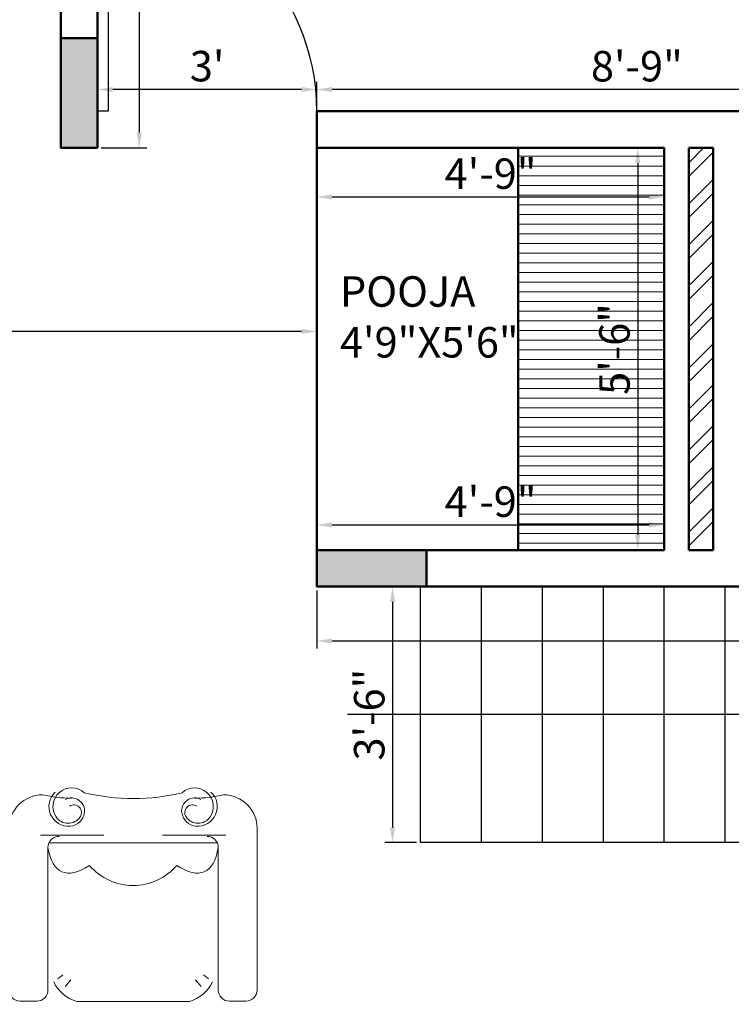
# Model space of a CAD drawing. Units: inches. Extents: x 3064 to 19385, y 846 to 15425.
# Tile 85 of 108: x 7228 to 7345, y 1112 to 1273. Entities that reach past the tile are written whole.
import ezdxf

# ---------------------------------------------------------------- set-up
doc = ezdxf.new("R2010")
doc.units = ezdxf.units.IN
for name, color, linetype, lineweight in [('A-ANNO-DIMS', 2, 'Continuous', 18), ('A-AREA-IDEN', 3, 'Continuous', 18), ('A-COLS', 1, 'Continuous', 35), ('A-DOOR', 3, 'Continuous', 25), ('A-FLOR-STRS', 2, 'Continuous', 25), ('A-FURN', 8, 'Continuous', 18), ('A-FURN-PATT', 252, 'Continuous', 13), ('A-WALL', 7, 'Continuous', 50)]:
    doc.layers.add(name, color=color, linetype=linetype, lineweight=lineweight)
doc.styles.get("Standard").update_dxf_attribs({"font": 'arial.ttf'})
doc.dimstyles.new('ISO-25', dxfattribs={"dimtxt": 9, "dimasz": 2.5, "dimexe": 1.25, "dimexo": 0.625, "dimtad": 1, "dimdec": 1, "dimlunit": 3, "dimtxsty": 'Standard', "dimcen": 2.5, "dimadec": 0, "dimazin": 0, "dimtfac": 1, "dimtdec": 1, "dimtmove": 0, "dimatfit": 3, "dimfxl": 1, "dimarcsym": 0})

# ---------------------------------------------------------------- blocks, each defined once
blk = doc.blocks.new('*U3')
for p, q in [((0, 0), (0, -6)), ((36, 0), (36, -6))]:
    blk.add_line(p, q)
blk.add_lwpolyline([(0, 0), (0, 36), (1.75, 36), (1.75, 0)], close=True)
blk.add_arc((0, 0), 36, 0, 90)
blk = doc.blocks.new('*D281')
at = {"layer": 'A-ANNO-DIMS', "color": 0, "lineweight": -2, "transparency": 16777216}
for p, q in [((7276.71, 1258.96), (7276.71, 1263.17)), ((7379.21, 1261.92), (7279.21, 1261.92)), ((7381.71, 1258.96), (7381.71, 1263.17))]:
    blk.add_line(p, q, dxfattribs=at)
at = {"layer": 'A-ANNO-DIMS', "color": 0, "transparency": 16777216}
for points in [[(7279.21, 1262.33), (7279.21, 1261.5), (7276.71, 1261.92)], [(7379.21, 1262.33), (7379.21, 1261.5), (7381.71, 1261.92)]]:
    blk.add_solid(points, dxfattribs=at)
at = {"layer": 'Defpoints', "color": 0, "transparency": 16777216}
for p in [(7276.71, 1261.92), (7276.71, 1258.34), (7381.71, 1258.34)]:
    blk.add_point(p, dxfattribs=at)
at = {"layer": 'A-ANNO-DIMS', "color": 0, "transparency": 16777216, "insert": (7329.21, 1265.09), "char_height": 5, "attachment_point": 5}
blk.add_mtext('8\'-9"', dxfattribs=at)
blk = doc.blocks.new('*D282')
at = {"layer": 'A-ANNO-DIMS', "color": 0, "lineweight": -2, "transparency": 16777216}
for p, q in [((7240.71, 1258.96), (7240.71, 1263.17)), ((7274.21, 1261.92), (7243.21, 1261.92)), ((7276.71, 1258.96), (7276.71, 1263.17))]:
    blk.add_line(p, q, dxfattribs=at)
at = {"layer": 'A-ANNO-DIMS', "color": 0, "transparency": 16777216}
for points in [[(7243.21, 1262.33), (7243.21, 1261.5), (7240.71, 1261.92)], [(7274.21, 1262.33), (7274.21, 1261.5), (7276.71, 1261.92)]]:
    blk.add_solid(points, dxfattribs=at)
at = {"layer": 'Defpoints', "color": 0, "transparency": 16777216}
for p in [(7240.71, 1261.92), (7240.71, 1258.34), (7276.71, 1258.34)]:
    blk.add_point(p, dxfattribs=at)
at = {"layer": 'A-ANNO-DIMS', "color": 0, "transparency": 16777216, "insert": (7258.71, 1265.1), "char_height": 5, "attachment_point": 5}
blk.add_mtext("3'", dxfattribs=at)
blk = doc.blocks.new('*D275')
at = {"layer": 'A-ANNO-DIMS', "color": 0, "lineweight": -2, "transparency": 16777216}
for p, q in [((7241.33, 1390.34), (7248.82, 1390.34)), ((7247.57, 1387.84), (7247.57, 1254.84)), ((7241.33, 1252.34), (7248.82, 1252.34))]:
    blk.add_line(p, q, dxfattribs=at)
at = {"layer": 'A-ANNO-DIMS', "color": 0, "transparency": 16777216}
for points in [[(7247.15, 1387.84), (7247.99, 1387.84), (7247.57, 1390.34)], [(7247.15, 1254.84), (7247.99, 1254.84), (7247.57, 1252.34)]]:
    blk.add_solid(points, dxfattribs=at)
at = {"layer": 'Defpoints', "color": 0, "transparency": 16777216}
for p in [(7240.71, 1390.34), (7240.71, 1252.34), (7247.57, 1252.34)]:
    blk.add_point(p, dxfattribs=at)
at = {"layer": 'A-ANNO-DIMS', "color": 0, "transparency": 16777216, "insert": (7244.39, 1321.34), "char_height": 5, "attachment_point": 5, "rotation": 90}
blk.add_mtext('11\'-6"', dxfattribs=at)
blk = doc.blocks.new('*D276')
at = {"layer": 'A-ANNO-DIMS', "color": 0, "lineweight": -2, "transparency": 16777216}
for p, q in [((7276.71, 1251.71), (7276.71, 1243.03)), ((7333.71, 1251.71), (7333.71, 1243.03)), ((7279.21, 1244.28), (7331.21, 1244.28))]:
    blk.add_line(p, q, dxfattribs=at)
at = {"layer": 'A-ANNO-DIMS', "color": 0, "transparency": 16777216}
for points in [[(7279.21, 1244.7), (7279.21, 1243.86), (7276.71, 1244.28)], [(7331.21, 1244.7), (7331.21, 1243.86), (7333.71, 1244.28)]]:
    blk.add_solid(points, dxfattribs=at)
at = {"layer": 'Defpoints', "color": 0, "transparency": 16777216}
for p in [(7276.71, 1252.34), (7333.71, 1252.34), (7333.71, 1244.28)]:
    blk.add_point(p, dxfattribs=at)
at = {"layer": 'A-ANNO-DIMS', "color": 0, "transparency": 16777216, "insert": (7305.21, 1247.46), "char_height": 5, "attachment_point": 5}
blk.add_mtext('4\'-9"', dxfattribs=at)
blk = doc.blocks.new('*D277')
at = {"layer": 'A-ANNO-DIMS', "color": 0, "lineweight": -2, "transparency": 16777216}
for p, q in [((7333.08, 1252.34), (7328.11, 1252.34)), ((7329.36, 1249.84), (7329.36, 1188.84)), ((7333.08, 1186.34), (7328.11, 1186.34))]:
    blk.add_line(p, q, dxfattribs=at)
at = {"layer": 'A-ANNO-DIMS', "color": 0, "transparency": 16777216}
for points in [[(7328.94, 1249.84), (7329.77, 1249.84), (7329.36, 1252.34)], [(7328.94, 1188.84), (7329.77, 1188.84), (7329.36, 1186.34)]]:
    blk.add_solid(points, dxfattribs=at)
at = {"layer": 'Defpoints', "color": 0, "transparency": 16777216}
for p in [(7333.71, 1252.34), (7329.36, 1186.34), (7333.71, 1186.34)]:
    blk.add_point(p, dxfattribs=at)
at = {"layer": 'A-ANNO-DIMS', "color": 0, "transparency": 16777216, "insert": (7326.18, 1219.34), "char_height": 5, "attachment_point": 5, "rotation": 90}
blk.add_mtext('5\'-6"', dxfattribs=at)
blk = doc.blocks.new('*D283')
at = {"layer": 'A-ANNO-DIMS', "color": 0, "lineweight": -2, "transparency": 16777216}
for p, q in [((7276.71, 1186.96), (7276.71, 1191.72)), ((7333.71, 1186.96), (7333.71, 1191.72)), ((7279.21, 1190.47), (7331.21, 1190.47))]:
    blk.add_line(p, q, dxfattribs=at)
at = {"layer": 'A-ANNO-DIMS', "color": 0, "transparency": 16777216}
for points in [[(7279.21, 1190.88), (7279.21, 1190.05), (7276.71, 1190.47)], [(7331.21, 1190.88), (7331.21, 1190.05), (7333.71, 1190.47)]]:
    blk.add_solid(points, dxfattribs=at)
at = {"layer": 'Defpoints', "color": 0, "transparency": 16777216}
for p in [(7333.71, 1190.47), (7276.71, 1186.34), (7333.71, 1186.34)]:
    blk.add_point(p, dxfattribs=at)
at = {"layer": 'A-ANNO-DIMS', "color": 0, "transparency": 16777216, "insert": (7305.21, 1193.64), "char_height": 5, "attachment_point": 5}
blk.add_mtext('4\'-9"', dxfattribs=at)
blk = doc.blocks.new('*D238')
at = {"layer": 'A-ANNO-DIMS', "color": 0, "lineweight": -2, "transparency": 16777216}
for p, q in [((7276.71, 1179.71), (7276.71, 1170.17)), ((7435.71, 1179.71), (7435.71, 1170.17)), ((7279.21, 1171.42), (7433.21, 1171.42))]:
    blk.add_line(p, q, dxfattribs=at)
at = {"layer": 'A-ANNO-DIMS', "color": 0, "transparency": 16777216}
for points in [[(7279.21, 1171.84), (7279.21, 1171.01), (7276.71, 1171.42)], [(7433.21, 1171.84), (7433.21, 1171.01), (7435.71, 1171.42)]]:
    blk.add_solid(points, dxfattribs=at)
at = {"layer": 'Defpoints', "color": 0, "transparency": 16777216}
for p in [(7276.71, 1180.34), (7435.71, 1180.34), (7435.71, 1171.42)]:
    blk.add_point(p, dxfattribs=at)
at = {"layer": 'A-ANNO-DIMS', "color": 0, "transparency": 16777216, "insert": (7356.21, 1174.6), "char_height": 5, "attachment_point": 5}
blk.add_mtext('13\'-3"', dxfattribs=at)
blk = doc.blocks.new('*D239')
at = {"layer": 'A-ANNO-DIMS', "color": 0, "lineweight": -2, "transparency": 16777216}
for p, q in [((7105.71, 1222.85), (7105.71, 1223.48)), ((7276.71, 1222.85), (7276.71, 1223.48)), ((7274.21, 1222.23), (7108.21, 1222.23))]:
    blk.add_line(p, q, dxfattribs=at)
at = {"layer": 'A-ANNO-DIMS', "color": 0, "transparency": 16777216}
for points in [[(7108.21, 1222.64), (7108.21, 1221.81), (7105.71, 1222.23)], [(7274.21, 1222.64), (7274.21, 1221.81), (7276.71, 1222.23)]]:
    blk.add_solid(points, dxfattribs=at)
at = {"layer": 'Defpoints', "color": 0, "transparency": 16777216}
for p in [(7105.71, 1222.23), (7105.71, 1222.23), (7276.71, 1222.23)]:
    blk.add_point(p, dxfattribs=at)
at = {"layer": 'A-ANNO-DIMS', "color": 0, "transparency": 16777216, "insert": (7191.21, 1225.4), "char_height": 5, "attachment_point": 5}
blk.add_mtext('14\'-3"', dxfattribs=at)
blk = doc.blocks.new('*D260')
at = {"layer": 'A-ANNO-DIMS', "color": 0, "lineweight": -2, "transparency": 16777216}
for p, q in [((7293.08, 1180.34), (7287.88, 1180.34)), ((7289.13, 1177.84), (7289.13, 1140.84)), ((7293.08, 1138.34), (7287.88, 1138.34))]:
    blk.add_line(p, q, dxfattribs=at)
at = {"layer": 'A-ANNO-DIMS', "color": 0, "transparency": 16777216}
for points in [[(7288.71, 1177.84), (7289.54, 1177.84), (7289.13, 1180.34)], [(7288.71, 1140.84), (7289.54, 1140.84), (7289.13, 1138.34)]]:
    blk.add_solid(points, dxfattribs=at)
at = {"layer": 'Defpoints', "color": 0, "transparency": 16777216}
for p in [(7293.71, 1180.34), (7289.13, 1138.34), (7293.71, 1138.34)]:
    blk.add_point(p, dxfattribs=at)
at = {"layer": 'A-ANNO-DIMS', "color": 0, "transparency": 16777216, "insert": (7285.95, 1159.34), "char_height": 5, "attachment_point": 5, "rotation": 90}
blk.add_mtext('3\'-6"', dxfattribs=at)
blk = doc.blocks.new('sofa-34')
at = {"color": 0, "linetype": 'ByBlock'}
for p, q in [((-0.026, 0.9238), (-0.1, 0.9238)), ((0.657, 0.9252), (0.1531, 0.9252)), ((0.8361, 0.9238), (0.9101, 0.9238)), ((-0.15, 0.15), (-0.15, 0.8738)), ((0.024, 0.2361), (0.024, 0.8738)), ((0.05, 0.8375), (0.05, 0.8379)), ((0.1006, 0.8574), (0.1265, 0.8286)), ((0.7096, 0.8574), (0.6837, 0.8286)), ((0.7601, 0.8375), (0.7601, 0.8379)), ((0.7602, 0.8375), (0.7601, 0.8379)), ((0.7861, 0.2361), (0.7861, 0.8738)), ((0.9601, 0.15), (0.9601, 0.8738)), ((0.0903, 0.8062), (0.0682, 0.8242)), ((0.7199, 0.8062), (0.742, 0.8242)), ((-0.01, 0.1801), (0.2738, 0.1801)), ((0.0289, 0.2145), (0.7812, 0.2145)), ((0.8201, 0.1801), (0.5364, 0.1801))]:
    blk.add_line(p, q, dxfattribs=at)
blk.add_arc((0.4051, 0.1479), 0.2579, 40.7983, 139.2017, dxfattribs=at)
at = {"color": 0, "linetype": 'ByBlock', "extrusion": (0, 0, -1)}
for centre, major_axis, ratio, start_param, end_param in [((-0.1, 0.8738), (0.0354, 0.0354), 1, 3.926992, 5.497787), ((-0.026, 0.8738), (-0.0354, 0.0354), 1, 0.785398, 2.356196), ((0.1997, 0.7661), (0.1173, 0.1173), 1, 4.372209, 5.213218), ((0.6105, 0.7661), (0.1173, 0.1173), 1, -0.500829, 0.34018), ((0.5004, -0.5869), (-0.4145, 0.931), 0.264583, -0.381915, 0.387685), ((0.074, 0.2361), (-0.0354, 0.0354), 1, 3.926991, 5.497788), ((0, 0.15), (0.1061, 0.1061), 1, 2.356194, 3.926992), ((0.1167, 0.0525), (-0.0624, 0.0624), 1, 4.675944, 7.152385), ((0.1183, 0.0712), (0.0491, 0.0491), 1, -0.701597, 0.659711), ((0.1299, 0.0524), (-0.059, 0.059), 1, 3.186406, 6.094039), ((0.1144, 0.0629), (-0.0458, 0.0458), 1, 6.094039, 8.043134), ((0.1392, 0.0798), (0.0245, 0.0245), 1, 0.189152, 2.952444), ((0.1292, 0.0726), (-0.0414, 0.0414), 1, 2.230507, 4.423483), ((0.179, -0.6576), (-0.2506, 0.635), 0.885019, 0.124301, 0.339591), ((0.3517, -0.5578), (0.7346, 0.1067), 0.76838, 4.597815, 5.20076)]:
    blk.add_ellipse(centre, major_axis=major_axis, ratio=ratio, start_param=start_param, end_param=end_param, dxfattribs=at)
at = {"color": 0, "linetype": 'ByBlock'}
for centre, major_axis, ratio, start_param, end_param in [((0.8361, 0.8738), (0.0354, 0.0354), 1, 0.785398, 2.356196), ((0.9101, 0.8738), (-0.0354, 0.0354), 1, 3.926992, 5.497787), ((0.3097, -0.5869), (0.4145, 0.931), 0.264583, -0.381915, 0.387685), ((0.7361, 0.2361), (0.0354, 0.0354), 1, 3.926991, 5.497788), ((0.6918, 0.0712), (-0.0491, 0.0491), 1, -0.701597, 0.659711), ((0.6934, 0.0525), (0.0624, 0.0624), 1, 4.675944, 7.152385), ((0.8101, 0.15), (-0.1061, 0.1061), 1, 2.356194, 3.926992), ((0.6802, 0.0524), (0.059, 0.059), 1, 3.186406, 6.094039), ((0.6709, 0.0798), (-0.0245, 0.0245), 1, 0.189152, 2.952444), ((0.6958, 0.0629), (0.0458, 0.0458), 1, 6.094039, 8.043134), ((0.6809, 0.0726), (0.0414, 0.0414), 1, 2.230507, 4.423483), ((0.6312, -0.6576), (0.2506, 0.635), 0.885019, 0.124301, 0.339591)]:
    blk.add_ellipse(centre, major_axis=major_axis, ratio=ratio, start_param=start_param, end_param=end_param, dxfattribs=at)

msp = doc.modelspace()

# ---------------------------------------------------------------- hatches: boundary and pattern name
at = {"layer": 'A-COLS'}
h = msp.add_hatch(color=256, dxfattribs=at)
h.dxf.hatch_style = 1
h.paths.add_polyline_path([(7234.71, 1252.34), (7240.71, 1252.34), (7240.71, 1270.34), (7234.71, 1270.34)])
h = msp.add_hatch(color=256, dxfattribs=at)
h.dxf.hatch_style = 1
h.paths.add_polyline_path([(7294.71, 1180.34), (7294.71, 1186.34), (7276.71, 1186.34), (7276.71, 1180.34)])
at = {"layer": 'A-FURN-PATT'}
h = msp.add_hatch(dxfattribs=at)
h.set_pattern_fill('ANSI31', color=256, scale=0.5, angle=135)
h.set_pattern_definition([(180, (1784.0376, -1e-11), (-1e-16, -1.5875), [])])
h.paths.add_polyline_path([(7309.71, 1186.34), (7333.71, 1186.34), (7333.71, 1252.34), (7309.71, 1252.34)])
h = msp.add_hatch(dxfattribs=at)
h.set_pattern_fill('ANSI32', color=256, scale=0.5)
h.set_pattern_definition([(45, (1784.0376, 0), (-3.367596, 3.367596), []), (45, (1786.2827, 0), (-3.367596, 3.367596), [])])
h.paths.add_polyline_path([(7337.71, 1186.34), (7341.71, 1186.34), (7341.71, 1252.34), (7337.71, 1252.34)])

# ---------------------------------------------------------------- linework, layer by layer
at = {"layer": 'A-FLOR-STRS'}
for p, q in [((7293.71, 1138.34), (7293.71, 1180.34)), ((7303.71, 1138.34), (7303.71, 1180.34)), ((7313.71, 1138.34), (7313.71, 1180.34)), ((7323.71, 1138.34), (7323.71, 1180.34)), ((7333.71, 1138.34), (7333.71, 1180.34)), ((7343.71, 1138.34), (7343.71, 1180.34)), ((7393.71, 1138.34), (7293.71, 1138.34))]:
    msp.add_line(p, q, dxfattribs=at)
msp.add_lwpolyline([(7301.19, 1003.34), (7408.71, 1003.34, 0.414214), (7414.71, 1009.34), (7414.71, 1153.34, 0.414214), (7408.71, 1159.34), (7281.71, 1159.34)], format="xyb", dxfattribs=at)
at = {"layer": 'A-WALL'}
for p, q in [((7234.71, 1390.34), (7234.71, 1252.34)), ((7240.71, 1390.34), (7240.71, 1252.34)), ((7381.71, 1258.34), (7276.71, 1258.34)), ((7276.71, 1258.34), (7276.71, 1180.34)), ((7276.71, 1258.34), (7276.71, 1180.34)), ((7240.71, 1252.34), (7234.71, 1252.34)), ((7333.71, 1252.34), (7276.71, 1252.34)), ((7309.71, 1252.34), (7309.71, 1186.34)), ((7333.71, 1252.34), (7333.71, 1186.34)), ((7341.71, 1252.34), (7337.71, 1252.34)), ((7337.71, 1252.34), (7337.71, 1186.34)), ((7341.71, 1186.34), (7341.71, 1252.34)), ((7333.71, 1186.34), (7276.71, 1186.34)), ((7341.71, 1186.34), (7337.71, 1186.34)), ((7435.71, 1180.34), (7276.71, 1180.34))]:
    msp.add_line(p, q, dxfattribs=at)
for points in [[(7240.71, 1252.34), (7240.71, 1270.34), (7234.71, 1270.34), (7234.71, 1252.34)], [(7294.71, 1186.34), (7276.71, 1186.34), (7276.71, 1180.34), (7294.71, 1180.34)]]:
    msp.add_lwpolyline(points, close=True, dxfattribs=at)

# ---------------------------------------------------------------- block references
at = {"layer": 'A-DOOR'}
msp.add_blockref('*U3', (7240.71, 1258.34), dxfattribs=at)
at = {"layer": 'A-FURN', "xscale": -36.66436083614781, "yscale": 36.66436083614781, "zscale": 36.66436083614781, "rotation": 180}
msp.add_blockref('sofa-34', (7231.71, 1146.18), dxfattribs=at)

# ---------------------------------------------------------------- texts
at = {"layer": 'A-AREA-IDEN', "insert": (7280.5, 1231.27), "char_height": 5, "attachment_point": 1}
msp.add_mtext_dynamic_manual_height_columns('POOJA\\P4\'9"X5\'6"', width=67.5924, gutter_width=12.5, heights=[0], dxfattribs=at)

# ---------------------------------------------------------------- dimensions: what is measured, and where the dimension line sits
at = {"layer": 'A-ANNO-DIMS'}
for base, p1, p2, picture, middle in [((7247.57, 1252.34), (7240.71, 1390.34), (7240.71, 1252.34), '*D275', (7244.39, 1321.34)), ((7329.36, 1186.34), (7333.71, 1252.34), (7333.71, 1186.34), '*D277', (7326.18, 1219.34)), ((7289.13, 1138.34), (7293.71, 1180.34), (7293.71, 1138.34), '*D260', (7285.95, 1159.34))]:
    dim = msp.add_linear_dim(base=base, p1=p1, p2=p2, angle=90, dimstyle='ISO-25', override={"dimtxt": 5, "dimclrd": 0, "dimclre": 0, "dimclrt": 0}, dxfattribs=at)
    dim.commit()
    dim.dimension.update_dxf_attribs({"geometry": picture, "text_midpoint": middle})
for base, p1, p2, override, picture, middle in [((7240.71, 1261.92), (7276.71, 1258.34), (7240.71, 1258.34), {"dimtxt": 5, "dimclrd": 0, "dimclre": 0, "dimclrt": 0, "dimtmove": 1}, '*D282', (7258.71, 1265.1)), ((7276.71, 1261.92), (7381.71, 1258.34), (7276.71, 1258.34), {"dimtxt": 5, "dimclrd": 0, "dimclre": 0, "dimclrt": 0, "dimtmove": 1}, '*D281', (7329.21, 1265.09)), ((7333.71, 1244.28), (7276.71, 1252.34), (7333.71, 1252.34), {"dimtxt": 5, "dimclrd": 0, "dimclre": 0, "dimclrt": 0}, '*D276', (7305.21, 1247.46)), ((7105.71, 1222.23), (7276.71, 1222.23), (7105.71, 1222.23), {"dimtxt": 5, "dimclrd": 0, "dimclre": 0, "dimclrt": 0}, '*D239', (7191.21, 1225.4)), ((7333.71, 1190.47), (7276.71, 1186.34), (7333.71, 1186.34), {"dimtxt": 5, "dimclrd": 0, "dimclre": 0, "dimclrt": 0}, '*D283', (7305.21, 1193.64)), ((7435.71, 1171.42), (7276.71, 1180.34), (7435.71, 1180.34), {"dimtxt": 5, "dimclrd": 0, "dimclre": 0, "dimclrt": 0}, '*D238', (7356.21, 1174.6))]:
    dim = msp.add_linear_dim(base=base, p1=p1, p2=p2, dimstyle='ISO-25', override=override, dxfattribs=at)
    dim.commit()
    dim.dimension.update_dxf_attribs({"geometry": picture, "text_midpoint": middle})

doc.saveas('drawing.dxf')
